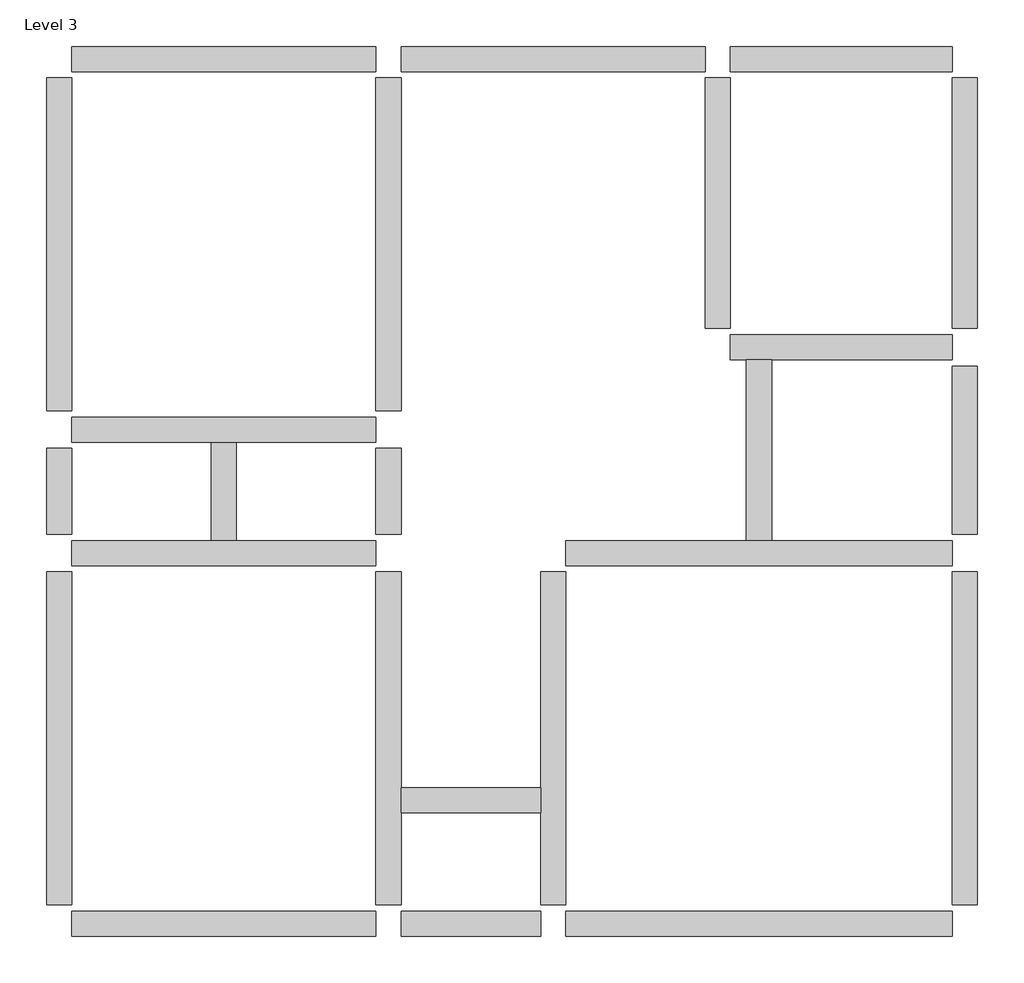
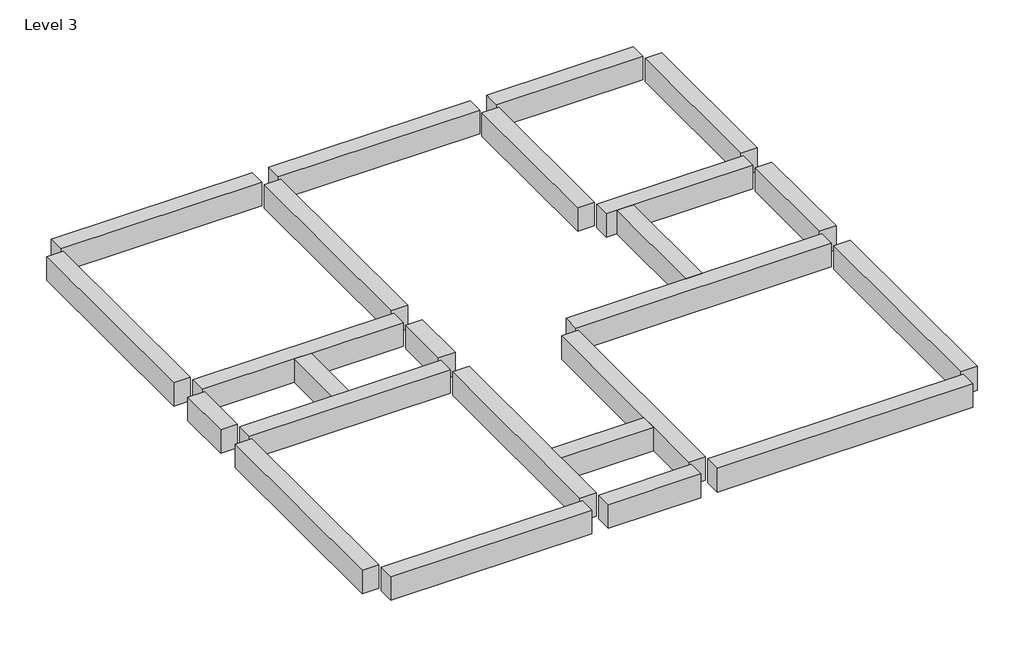
# One storey: 14 beams.
"""IFC4 building model written with IfcOpenShell, lengths in millimetres."""

from ifc_helpers import new_model, si_unit, frame, origin, place, context, project, spatial, polyline, outline, extrude, faceted_brep, element, save

model = new_model("IFC4")

# Units and contexts
model_context = context("Model", 3, world=origin())
ifc_project = project(units=[si_unit("LENGTHUNIT", "METRE", prefix="MILLI")], contexts=[model_context])

# Site, building, storey
site = spatial("IfcSite", under=ifc_project)
building = spatial("IfcBuilding", under=site)
storey = spatial("IfcBuildingStorey", under=building, Name="Level 3", Elevation=6096.0)

# Beams
placement = place(None, origin())
element("IfcBeam", 1, ObjectType="Concrete-Rectangular Beam : 12 x 24", at=placement, inside=storey, context=model_context, shape_type="SweptSolid", body=[
    extrude(outline(polyline([(-4459.6215379, 8530.2267522), (-4459.6215379, 8225.4267522), (-7154.8215379, 8225.4267522), (-7154.8215379, 8530.2267522), (-4459.6215379, 8530.2267522)])), frame((0.0, 0.0, 5638.8), z_axis=(0.0, 0.0, 1.0), x_axis=(1.0, 0.0, 0.0)), (0.0, 0.0, 1.0), 457.2),
    extrude(outline(polyline([(-15154.8215379, 8225.4267522), (-15154.8215379, 8530.2267522), (-11459.6215379, 8530.2267522), (-11459.6215379, 8225.4267522), (-15154.8215379, 8225.4267522)])), frame((0.0, 0.0, 5638.8), z_axis=(0.0, 0.0, 1.0), x_axis=(1.0, 0.0, 0.0)), (0.0, 0.0, 1.0), 457.2),
    extrude(outline(polyline([(-11154.8215379, 8225.4267522), (-11154.8215379, 8530.2267522), (-7459.6215379, 8530.2267522), (-7459.6215379, 8225.4267522), (-11154.8215379, 8225.4267522)])), frame((0.0, 0.0, 5638.8), z_axis=(0.0, 0.0, 1.0), x_axis=(1.0, 0.0, 0.0)), (0.0, 0.0, 1.0), 457.2),
])
element("IfcBeam", 2, ObjectType="Concrete-Rectangular Beam : 12 x 24", at=placement, inside=storey, context=model_context, shape_type="SweptSolid", body=[
    extrude(outline(polyline([(-4154.8215379, -1893.5732478), (-4459.6215379, -1893.5732478), (-4459.6215379, 2149.2267522), (-4154.8215379, 2149.2267522), (-4154.8215379, -1893.5732478)])), frame((0.0, 0.0, 5638.8), z_axis=(0.0, 0.0, 1.0), x_axis=(1.0, 0.0, 0.0)), (0.0, 0.0, 1.0), 457.2),
    extrude(outline(polyline([(-4459.6215379, 8149.2267522), (-4154.8215379, 8149.2267522), (-4154.8215379, 5106.4267522), (-4459.6215379, 5106.4267522), (-4459.6215379, 8149.2267522)])), frame((0.0, 0.0, 5638.8), z_axis=(0.0, 0.0, 1.0), x_axis=(1.0, 0.0, 0.0)), (0.0, 0.0, 1.0), 457.2),
    extrude(outline(polyline([(-4154.8215379, 2606.4267522), (-4459.6215379, 2606.4267522), (-4459.6215379, 4649.2267522), (-4154.8215379, 4649.2267522), (-4154.8215379, 2606.4267522)])), frame((0.0, 0.0, 5638.8), z_axis=(0.0, 0.0, 1.0), x_axis=(1.0, 0.0, 0.0)), (0.0, 0.0, 1.0), 457.2),
])
element("IfcBeam", 3, ObjectType="Concrete-Rectangular Beam : 12 x 24", at=placement, inside=storey, context=model_context, shape_type="SweptSolid", body=[
    extrude(outline(polyline([(-15154.8215379, -2274.5732478), (-15154.8215379, -1969.7732478), (-11459.6215379, -1969.7732478), (-11459.6215379, -2274.5732478), (-15154.8215379, -2274.5732478)])), frame((0.0, 0.0, 5638.8), z_axis=(0.0, 0.0, 1.0), x_axis=(1.0, 0.0, 0.0)), (0.0, 0.0, 1.0), 457.2),
    extrude(outline(polyline([(-4459.6215379, -1969.7732478), (-4459.6215379, -2274.5732478), (-9154.8215379, -2274.5732478), (-9154.8215379, -1969.7732478), (-4459.6215379, -1969.7732478)])), frame((0.0, 0.0, 5638.8), z_axis=(0.0, 0.0, 1.0), x_axis=(1.0, 0.0, 0.0)), (0.0, 0.0, 1.0), 457.2),
    extrude(outline(polyline([(-11154.8215379, -2274.5732478), (-11154.8215379, -1969.7732478), (-9459.6215379, -1969.7732478), (-9459.6215379, -2274.5732478), (-11154.8215379, -2274.5732478)])), frame((0.0, 0.0, 5638.8), z_axis=(0.0, 0.0, 1.0), x_axis=(1.0, 0.0, 0.0)), (0.0, 0.0, 1.0), 457.2),
])
element("IfcBeam", 4, ObjectType="Concrete-Rectangular Beam : 12 x 24", at=placement, inside=storey, context=model_context, shape_type="SweptSolid", body=[
    extrude(outline(polyline([(-15459.6215379, 8149.2267522), (-15154.8215379, 8149.2267522), (-15154.8215379, 4106.4267522), (-15459.6215379, 4106.4267522), (-15459.6215379, 8149.2267522)])), frame((0.0, 0.0, 5638.8), z_axis=(0.0, 0.0, 1.0), x_axis=(1.0, 0.0, 0.0)), (0.0, 0.0, 1.0), 457.2),
    extrude(outline(polyline([(-15154.8215379, -1893.5732478), (-15459.6215379, -1893.5732478), (-15459.6215379, 2149.2267522), (-15154.8215379, 2149.2267522), (-15154.8215379, -1893.5732478)])), frame((0.0, 0.0, 5638.8), z_axis=(0.0, 0.0, 1.0), x_axis=(1.0, 0.0, 0.0)), (0.0, 0.0, 1.0), 457.2),
    extrude(outline(polyline([(-15459.6215379, 3649.2267522), (-15154.8215379, 3649.2267522), (-15154.8215379, 2606.4267522), (-15459.6215379, 2606.4267522), (-15459.6215379, 3649.2267522)])), frame((0.0, 0.0, 5638.8), z_axis=(0.0, 0.0, 1.0), x_axis=(1.0, 0.0, 0.0)), (0.0, 0.0, 1.0), 457.2),
])
element("IfcBeam", 5, ObjectType="Concrete-Rectangular Beam : 12 x 24", at=placement, inside=storey, context=model_context, shape_type="Brep", body=[
    faceted_brep([(-11459.6215379, -1893.5732478, 6096.0), (-11154.8215379, -1893.5732478, 6096.0), (-11154.8215379, -774.5732478, 6096.0), (-11154.8215379, -469.7732478, 6096.0), (-11154.8215379, 2149.2267522, 6096.0), (-11459.6215379, 2149.2267522, 6096.0), (-11459.6215379, -1893.5732478, 5638.8), (-11459.6215379, 2149.2267522, 5638.8), (-11154.8215379, -1893.5732478, 5638.8), (-11154.8215379, 2149.2267522, 5638.8), (-11154.8215379, -469.7732478, 5638.8), (-11154.8215379, -774.5732478, 5638.8)], [[[0, 1, 2, 3, 4, 5]], [[6, 0, 5, 7]], [[8, 6, 7, 9, 10, 11]], [[1, 8, 11, 10, 9, 4, 3, 2]], [[1, 0, 6, 8]], [[5, 4, 9, 7]]]),
    faceted_brep([(-11459.6215379, 8149.2267522, 6096.0), (-11154.8215379, 8149.2267522, 6096.0), (-11154.8215379, 8149.2267522, 5638.8), (-11459.6215379, 8149.2267522, 5638.8), (-11154.8215379, 4106.4267522, 6096.0), (-11459.6215379, 4106.4267522, 6096.0), (-11459.6215379, 4106.4267522, 5638.8), (-11154.8215379, 4106.4267522, 5638.8)], [[[0, 1, 2, 3]], [[4, 5, 6, 7]], [[1, 0, 5, 4]], [[0, 3, 6, 5]], [[3, 2, 7, 6]], [[2, 1, 4, 7]]]),
    faceted_brep([(-11459.6215379, 3649.2267522, 6096.0), (-11154.8215379, 3649.2267522, 6096.0), (-11154.8215379, 3649.2267522, 5638.8), (-11459.6215379, 3649.2267522, 5638.8), (-11154.8215379, 2606.4267522, 6096.0), (-11459.6215379, 2606.4267522, 6096.0), (-11459.6215379, 2606.4267522, 5638.8), (-11154.8215379, 2606.4267522, 5638.8)], [[[0, 1, 2, 3]], [[4, 5, 6, 7]], [[1, 0, 5, 4]], [[0, 3, 6, 5]], [[3, 2, 7, 6]], [[2, 1, 4, 7]]]),
])
element("IfcBeam", 6, ObjectType="Concrete-Rectangular Beam : 12 x 24", at=placement, inside=storey, context=model_context, shape_type="Brep", body=[
    faceted_brep([(-9459.6215379, -1893.5732478, 6096.0), (-9154.8215379, -1893.5732478, 6096.0), (-9154.8215379, 2149.2267522, 6096.0), (-9459.6215379, 2149.2267522, 6096.0), (-9459.6215379, -469.7732478, 6096.0), (-9459.6215379, -774.5732478, 6096.0), (-9154.8215379, -1893.5732478, 5638.8), (-9154.8215379, 2149.2267522, 5638.8), (-9459.6215379, -1893.5732478, 5638.8), (-9459.6215379, -774.5732478, 5638.8), (-9459.6215379, -469.7732478, 5638.8), (-9459.6215379, 2149.2267522, 5638.8)], [[[0, 1, 2, 3, 4, 5]], [[1, 6, 7, 2]], [[6, 8, 9, 10, 11, 7]], [[8, 0, 5, 4, 3, 11, 10, 9]], [[1, 0, 8, 6]], [[3, 2, 7, 11]]]),
])
element("IfcBeam", 7, ObjectType="Concrete-Rectangular Beam : 12 x 24", at=placement, inside=storey, context=model_context, shape_type="Brep", body=[
    faceted_brep([(-9154.8215379, 2530.2267522, 6096.0), (-9154.8215379, 2225.4267522, 6096.0), (-4459.6215379, 2225.4267522, 6096.0), (-4459.6215379, 2530.2267522, 6096.0), (-6654.8215379, 2530.2267522, 6096.0), (-6959.6215379, 2530.2267522, 6096.0), (-9154.8215379, 2225.4267522, 5638.8), (-4459.6215379, 2225.4267522, 5638.8), (-9154.8215379, 2530.2267522, 5638.8), (-6959.6215379, 2530.2267522, 5638.8), (-6654.8215379, 2530.2267522, 5638.8), (-4459.6215379, 2530.2267522, 5638.8)], [[[0, 1, 2, 3, 4, 5]], [[1, 6, 7, 2]], [[6, 8, 9, 10, 11, 7]], [[3, 11, 10, 9, 8, 0, 5, 4]], [[0, 8, 6, 1]], [[3, 2, 7, 11]]]),
])
element("IfcBeam", 8, ObjectType="Concrete-Rectangular Beam : 12 x 24", at=placement, inside=storey, context=model_context, shape_type="SweptSolid", body=[
    extrude(outline(polyline([(-7459.6215379, 8149.2267522), (-7154.8215379, 8149.2267522), (-7154.8215379, 5106.4267522), (-7459.6215379, 5106.4267522), (-7459.6215379, 8149.2267522)])), frame((0.0, 0.0, 5638.8), z_axis=(0.0, 0.0, 1.0), x_axis=(1.0, 0.0, 0.0)), (0.0, 0.0, 1.0), 457.2),
])
element("IfcBeam", 9, ObjectType="Concrete-Rectangular Beam : 12 x 24", at=placement, inside=storey, context=model_context, shape_type="Brep", body=[
    faceted_brep([(-7154.8215379, 5030.2267522, 6096.0), (-7154.8215379, 4725.4267522, 6096.0), (-6959.6215379, 4725.4267522, 6096.0), (-6654.8215379, 4725.4267522, 6096.0), (-4459.6215379, 4725.4267522, 6096.0), (-4459.6215379, 5030.2267522, 6096.0), (-7154.8215379, 5030.2267522, 5638.8), (-4459.6215379, 5030.2267522, 5638.8), (-7154.8215379, 4725.4267522, 5638.8), (-4459.6215379, 4725.4267522, 5638.8), (-6654.8215379, 4725.4267522, 5638.8), (-6959.6215379, 4725.4267522, 5638.8)], [[[0, 1, 2, 3, 4, 5]], [[6, 0, 5, 7]], [[8, 6, 7, 9, 10, 11]], [[1, 8, 11, 10, 9, 4, 3, 2]], [[0, 6, 8, 1]], [[5, 4, 9, 7]]]),
])
element("IfcBeam", 10, ObjectType="Concrete-Rectangular Beam : 12 x 24", at=placement, inside=storey, context=model_context, shape_type="Brep", body=[
    faceted_brep([(-15154.8215379, 4030.2267522, 6096.0), (-15154.8215379, 3725.4267522, 6096.0), (-13459.6215379, 3725.4267522, 6096.0), (-13154.8215379, 3725.4267522, 6096.0), (-11459.6215379, 3725.4267522, 6096.0), (-11459.6215379, 4030.2267522, 6096.0), (-15154.8215379, 3725.4267522, 5638.8), (-13459.6215379, 3725.4267522, 5638.8), (-13154.8215379, 3725.4267522, 5638.8), (-11459.6215379, 3725.4267522, 5638.8), (-15154.8215379, 4030.2267522, 5638.8), (-11459.6215379, 4030.2267522, 5638.8)], [[[0, 1, 2, 3, 4, 5]], [[1, 6, 7, 8, 9, 4, 3, 2]], [[6, 10, 11, 9, 8, 7]], [[10, 0, 5, 11]], [[1, 0, 10, 6]], [[5, 4, 9, 11]]]),
])
element("IfcBeam", 11, ObjectType="Concrete-Rectangular Beam : 12 x 24", at=placement, inside=storey, context=model_context, shape_type="Brep", body=[
    faceted_brep([(-15154.8215379, 2530.2267522, 6096.0), (-15154.8215379, 2225.4267522, 6096.0), (-11459.6215379, 2225.4267522, 6096.0), (-11459.6215379, 2530.2267522, 6096.0), (-13154.8215379, 2530.2267522, 6096.0), (-13459.6215379, 2530.2267522, 6096.0), (-15154.8215379, 2530.2267522, 5638.8), (-11459.6215379, 2530.2267522, 5638.8), (-13154.8215379, 2530.2267522, 5638.8), (-13459.6215379, 2530.2267522, 5638.8), (-15154.8215379, 2225.4267522, 5638.8), (-11459.6215379, 2225.4267522, 5638.8)], [[[0, 1, 2, 3, 4, 5]], [[6, 0, 5, 4, 3, 7, 8, 9]], [[10, 6, 9, 8, 7, 11]], [[1, 10, 11, 2]], [[1, 0, 6, 10]], [[3, 2, 11, 7]]]),
])
element("IfcBeam", 12, ObjectType="Concrete-Rectangular Beam : 12 x 24", at=placement, inside=storey, context=model_context, shape_type="SweptSolid", body=[
    extrude(outline(polyline([(-13459.6215379, 3725.4267522), (-13154.8215379, 3725.4267522), (-13154.8215379, 2530.2267522), (-13459.6215379, 2530.2267522), (-13459.6215379, 3725.4267522)])), frame((0.0, 0.0, 5638.8), z_axis=(0.0, 0.0, 1.0), x_axis=(1.0, 0.0, 0.0)), (0.0, 0.0, 1.0), 457.2),
])
element("IfcBeam", 13, ObjectType="Concrete-Rectangular Beam : 12 x 24", at=placement, inside=storey, context=model_context, shape_type="SweptSolid", body=[
    extrude(outline(polyline([(-6654.8215379, 2530.2267522), (-6959.6215379, 2530.2267522), (-6959.6215379, 4725.4267522), (-6654.8215379, 4725.4267522), (-6654.8215379, 2530.2267522)])), frame((0.0, 0.0, 5638.8), z_axis=(0.0, 0.0, 1.0), x_axis=(1.0, 0.0, 0.0)), (0.0, 0.0, 1.0), 457.2),
])
element("IfcBeam", 14, ObjectType="Concrete-Rectangular Beam : 12 x 24", at=placement, inside=storey, context=model_context, shape_type="SweptSolid", body=[
    extrude(outline(polyline([(-11154.8215379, -774.5732478), (-11154.8215379, -469.7732478), (-9459.6215379, -469.7732478), (-9459.6215379, -774.5732478), (-11154.8215379, -774.5732478)])), frame((0.0, 0.0, 5638.8), z_axis=(0.0, 0.0, 1.0), x_axis=(1.0, 0.0, 0.0)), (0.0, 0.0, 1.0), 457.2),
])

save(model, "model.ifc")

# Revit data of these elements
# Type "Concrete-Rectangular Beam : 12 x 24"
#   Assembly Code = "B10"
#   Length [instance default] = 5' - 0"
#   b = 1' - 0"
#   h = 1' - 6"
#   Structural Material [instance default] = Concrete, Cast-in-Place gray
# Elements 1, 2, 3, 4, 5, 6, 7, 8, 9, 10, 11, 12, 13, 14 (IfcBeam, "Concrete-Rectangular Beam : 12 x 24")
#   Structural Material = Concrete, Cast-in-Place gray
#   Phase Created = New Construction
#   Materials on its faces: "Concrete, Cast-in-Place gray"
# Materials
#   "Concrete, Cast-in-Place gray": class "Concrete", colour RGB 192 192 192, transparency 0, Description = "Cast-in-place concrete", Cost = 0
